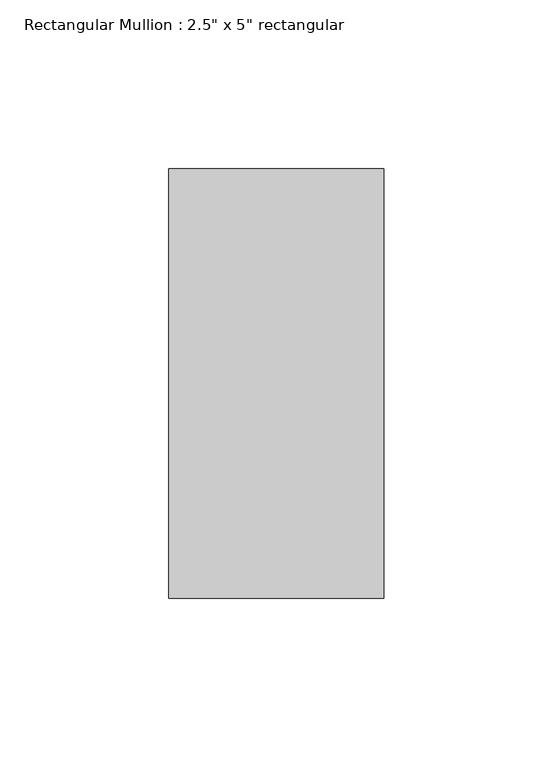
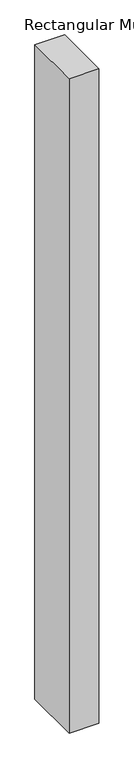
"""IFC4 building model written with IfcOpenShell, lengths in millimetres: member geometry."""

from ifc_helpers import new_model, si_unit, frame, origin, place, context, project, spatial, polyline, outline, extrude, source, transform, mapped, element, save


def member_d74100e1(model_context):
    return source(origin(), model_context, "Body", "SweptSolid", [
        extrude(outline(polyline([(0.0, 63.5), (0.0, -63.5), (-63.5, -63.5), (-63.5, 63.5), (0.0, 63.5)])), frame((0.0, 0.0, -1482.4314829), z_axis=(0.0, 0.0, 1.0), x_axis=(1.0, 0.0, 0.0)), (0.0, 0.0, 1.0), 1482.4314829),
    ])


if __name__ == "__main__":
    model = new_model("IFC4")
    model_context = context("Model", 3, world=origin())
    ifc_project = project(units=[si_unit("LENGTHUNIT", "METRE", prefix="MILLI")], contexts=[model_context])
    site = spatial("IfcSite", under=ifc_project)
    building = spatial("IfcBuilding", under=site)
    placement = place(None, origin())
    member_shape = member_d74100e1(model_context)
    element("IfcMember", 1, ObjectType="Rectangular Mullion : 2.5\" x 5\" rectangular", at=placement, inside=building, context=model_context, shape_type="MappedRepresentation", body=[
        mapped(member_shape, transform((0.0, 0.0, 0.0), x_axis=(1.0, 0.0, 0.0), y_axis=(0.0, 1.0, 0.0), z_axis=(0.0, 0.0, 1.0))),
    ])
    save(model, "model.ifc")

# Revit data of these elements
# Type "Rectangular Mullion : 2.5\" x 5\" rectangular"
#   built-in parameter 1007304 = 0.416667 (stored number, unit not read)
#   built-in parameter 1007301 = 0.104167 (stored number, unit not read)
#   built-in parameter 1007300 = 0.104167 (stored number, unit not read)
